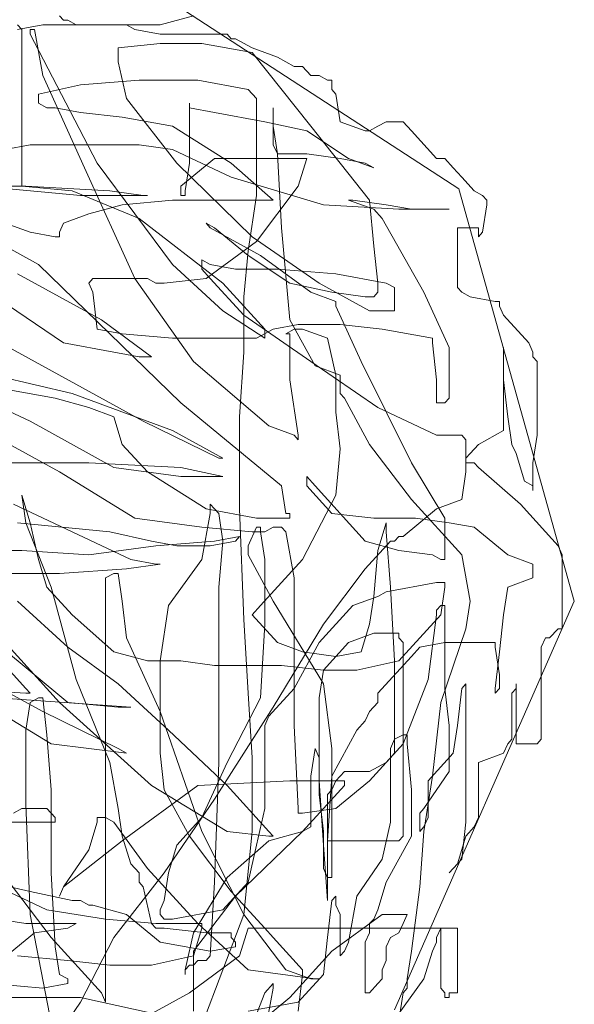
# Model space of a CAD drawing. Units: inches. Extents: x 1994 to 3075, y 3517 to 3950.
# Tile 41 of 58: x 1994.646332 to 1994.650517, y 3553.741889 to 3553.749313. Entities that reach past the tile are written whole.
import ezdxf

# ---------------------------------------------------------------- set-up
doc = ezdxf.new("R2010")
doc.units = ezdxf.units.IN
doc.layers.add('A-FURN-REFR', color=8, linetype='Continuous', lineweight=13)

msp = doc.modelspace()

# ---------------------------------------------------------------- linework, layer by layer
at = {"layer": 'A-FURN-REFR'}
for p, q in [((1994.6474175, 3553.7494858), (1994.6496449, 3553.7480373)), ((1994.6466639, 3553.7493078), (1994.6466323, 3553.7493426)), ((1994.6466955, 3553.7493078), (1994.6466639, 3553.7493078)), ((1994.6467587, 3553.7492731), (1994.6466955, 3553.7493078)), ((1994.6476438, 3553.7493426), (1994.647391, 3553.7492731)), ((1994.6463162, 3553.7492731), (1994.6463478, 3553.7492383)), ((1994.6465059, 3553.7492731), (1994.6463162, 3553.7492383)), ((1994.6463478, 3553.7492383), (1994.6463478, 3553.748057)), ((1994.6464111, 3553.7492383), (1994.6464427, 3553.7492383)), ((1994.6464111, 3553.7492037), (1994.6464111, 3553.7492383)), ((1994.6464427, 3553.7492383), (1994.6465059, 3553.7488909)), ((1994.647391, 3553.7492731), (1994.6465059, 3553.7492731)), ((1994.6471381, 3553.7492731), (1994.6467587, 3553.7492731)), ((1994.6472013, 3553.7492383), (1994.6471381, 3553.7492731)), ((1994.647391, 3553.7492037), (1994.6472013, 3553.7492383)), ((1994.6469168, 3553.7482307), (1994.6464111, 3553.7492037)), ((1994.6478967, 3553.7492037), (1994.647391, 3553.7492037)), ((1994.6479283, 3553.7491689), (1994.6478967, 3553.7492037)), ((1994.6479599, 3553.7491689), (1994.6479283, 3553.7491689)), ((1994.6480864, 3553.7490994), (1994.6479599, 3553.7491689)), ((1994.647391, 3553.7491341), (1994.6470749, 3553.7490994)), ((1994.6470749, 3553.7490994), (1994.6470749, 3553.7489951)), ((1994.647707, 3553.7491341), (1994.647391, 3553.7491341)), ((1994.6480864, 3553.7490646), (1994.647707, 3553.7491341)), ((1994.648276, 3553.7490299), (1994.6480864, 3553.7490994)), ((1994.6485289, 3553.7485087), (1994.6480864, 3553.7490646)), ((1994.6484025, 3553.7489604), (1994.648276, 3553.7490299)), ((1994.6470749, 3553.7489951), (1994.6471381, 3553.7487172)), ((1994.6484657, 3553.7489604), (1994.6484025, 3553.7489604)), ((1994.6485289, 3553.7488909), (1994.6484657, 3553.7489604)), ((1994.6465059, 3553.7488909), (1994.646822, 3553.7481959)), ((1994.6485921, 3553.7488909), (1994.6485289, 3553.7488909)), ((1994.6486553, 3553.7488562), (1994.6485921, 3553.7488909)), ((1994.6464743, 3553.7487519), (1994.6467904, 3553.7488214)), ((1994.6467904, 3553.7488214), (1994.6472329, 3553.7488562)), ((1994.6472329, 3553.7488562), (1994.6476754, 3553.7488562)), ((1994.6476754, 3553.7488562), (1994.6480548, 3553.7487867)), ((1994.6480548, 3553.7487867), (1994.648118, 3553.7487172)), ((1994.6486869, 3553.7488562), (1994.6486553, 3553.7488562)), ((1994.6486869, 3553.7487867), (1994.6486869, 3553.7488562)), ((1994.6487185, 3553.7487519), (1994.6486869, 3553.7487867)), ((1994.6464743, 3553.7486824), (1994.6464743, 3553.7487519)), ((1994.6471381, 3553.7487172), (1994.6475174, 3553.7482307)), ((1994.648118, 3553.7487172), (1994.648118, 3553.7479875)), ((1994.6487501, 3553.7485434), (1994.6487185, 3553.7487519)), ((1994.6465375, 3553.7486477), (1994.6464743, 3553.7486824)), ((1994.6466007, 3553.7486477), (1994.6465375, 3553.7486477)), ((1994.6467904, 3553.7486129), (1994.6466007, 3553.7486477)), ((1994.6476122, 3553.7486824), (1994.6476122, 3553.7482307)), ((1994.6476122, 3553.7486477), (1994.6476122, 3553.7486824)), ((1994.6478019, 3553.7486129), (1994.6476122, 3553.7486477)), ((1994.6482444, 3553.7486477), (1994.6482444, 3553.7483697)), ((1994.6482444, 3553.7485087), (1994.6482444, 3553.7486477)), ((1994.6471065, 3553.7485782), (1994.6467904, 3553.7486129)), ((1994.6474858, 3553.7485087), (1994.6471065, 3553.7485782)), ((1994.6481812, 3553.7485434), (1994.6478019, 3553.7486129)), ((1994.6479283, 3553.7482307), (1994.6474858, 3553.7485087)), ((1994.6484973, 3553.748474), (1994.6481812, 3553.7485434)), ((1994.648276, 3553.7483002), (1994.6482444, 3553.7485087)), ((1994.6489714, 3553.7479527), (1994.6485289, 3553.7485087)), ((1994.6489398, 3553.748474), (1994.6487501, 3553.7485434)), ((1994.6490347, 3553.7485087), (1994.6489714, 3553.748474)), ((1994.6490979, 3553.7485434), (1994.6490347, 3553.7485087)), ((1994.6492243, 3553.7485434), (1994.6490979, 3553.7485434)), ((1994.6492875, 3553.748474), (1994.6492243, 3553.7485434)), ((1994.6488134, 3553.7482654), (1994.6484973, 3553.748474)), ((1994.6489714, 3553.748474), (1994.6489398, 3553.748474)), ((1994.6494772, 3553.7482654), (1994.6492875, 3553.748474)), ((1994.6464111, 3553.7483697), (1994.6462214, 3553.7483349)), ((1994.6472329, 3553.7483697), (1994.6464111, 3553.7483697)), ((1994.6474858, 3553.7483349), (1994.6472329, 3553.7483697)), ((1994.6482444, 3553.7483697), (1994.648276, 3553.7483002)), ((1994.6479283, 3553.7481265), (1994.6474858, 3553.7483349)), ((1994.648276, 3553.7483002), (1994.6484973, 3553.7483002)), ((1994.6483076, 3553.7477443), (1994.648276, 3553.7483002)), ((1994.6484973, 3553.7483002), (1994.6487501, 3553.7482654)), ((1994.646822, 3553.7481959), (1994.6472013, 3553.747362)), ((1994.6474858, 3553.7474662), (1994.6469168, 3553.7482307)), ((1994.6475174, 3553.7482307), (1994.6480864, 3553.7476748)), ((1994.647549, 3553.748057), (1994.6478019, 3553.7482654)), ((1994.6476122, 3553.7482307), (1994.6475806, 3553.7480222)), ((1994.6478019, 3553.7482654), (1994.6484973, 3553.7482654)), ((1994.6482444, 3553.7479527), (1994.6479283, 3553.7482307)), ((1994.6484973, 3553.7482654), (1994.6484341, 3553.748057)), ((1994.6487501, 3553.7482654), (1994.6489398, 3553.7482307)), ((1994.649003, 3553.7481959), (1994.6488134, 3553.7482654)), ((1994.6489398, 3553.7482307), (1994.649003, 3553.7481959)), ((1994.6495404, 3553.7482654), (1994.6494772, 3553.7482654)), ((1994.6496036, 3553.7481959), (1994.6495404, 3553.7482654)), ((1994.6496669, 3553.7481265), (1994.6496036, 3553.7481959)), ((1994.6486237, 3553.747918), (1994.6479283, 3553.7481265)), ((1994.6497617, 3553.7480222), (1994.6496669, 3553.7481265)), ((1994.6451783, 3553.748057), (1994.6463794, 3553.748057)), ((1994.6467904, 3553.7479875), (1994.6460317, 3553.748057)), ((1994.6463478, 3553.748057), (1994.6467271, 3553.7480222)), ((1994.6463794, 3553.748057), (1994.6470116, 3553.7480222)), ((1994.647549, 3553.7479875), (1994.647549, 3553.748057)), ((1994.6484341, 3553.748057), (1994.648118, 3553.74764)), ((1994.6467271, 3553.7480222), (1994.6472329, 3553.7478137)), ((1994.6472961, 3553.7479875), (1994.6467904, 3553.7479875)), ((1994.6470116, 3553.7480222), (1994.6472645, 3553.7479875)), ((1994.6472645, 3553.7479875), (1994.6472961, 3553.7479875)), ((1994.6475806, 3553.7479875), (1994.647549, 3553.7479875)), ((1994.6475806, 3553.7480222), (1994.6475806, 3553.7479875)), ((1994.648118, 3553.7479875), (1994.6480548, 3553.7475705)), ((1994.6496449, 3553.7480373), (1994.6505167, 3553.7449295)), ((1994.6498249, 3553.7479875), (1994.6497617, 3553.7480222)), ((1994.6498565, 3553.7479527), (1994.6498249, 3553.7479875)), ((1994.6468536, 3553.7478485), (1994.6471065, 3553.747918)), ((1994.6471065, 3553.747918), (1994.6474858, 3553.7479527)), ((1994.6474858, 3553.7479527), (1994.6482444, 3553.7479527)), ((1994.6491927, 3553.7478832), (1994.6486237, 3553.747918)), ((1994.6488134, 3553.7479527), (1994.648845, 3553.7479527)), ((1994.649003, 3553.7478832), (1994.6488134, 3553.7479527)), ((1994.648845, 3553.7479527), (1994.6490979, 3553.747918)), ((1994.649003, 3553.7476053), (1994.6489714, 3553.7479527)), ((1994.6490979, 3553.747918), (1994.6492875, 3553.7478832)), ((1994.6498249, 3553.7477095), (1994.6498565, 3553.747918)), ((1994.6498565, 3553.747918), (1994.6498565, 3553.7479527)), ((1994.6457156, 3553.7478832), (1994.6464743, 3553.7474662)), ((1994.6466639, 3553.747779), (1994.6468536, 3553.7478485)), ((1994.6490663, 3553.7478137), (1994.649003, 3553.7478832)), ((1994.649572, 3553.7478832), (1994.6491927, 3553.7478832)), ((1994.6492875, 3553.7478832), (1994.649572, 3553.7478832)), ((1994.6462214, 3553.747779), (1994.6464111, 3553.7477095)), ((1994.6466323, 3553.7477095), (1994.6466639, 3553.747779)), ((1994.6472329, 3553.7478137), (1994.6478651, 3553.7473273)), ((1994.6477386, 3553.747779), (1994.6478019, 3553.7477443)), ((1994.6477703, 3553.7477443), (1994.6477386, 3553.747779)), ((1994.6493823, 3553.7472578), (1994.6490663, 3553.7478137)), ((1994.6464111, 3553.7477095), (1994.6466007, 3553.7476748)), ((1994.6466007, 3553.7476748), (1994.6466323, 3553.7476748)), ((1994.6466323, 3553.7476748), (1994.6466323, 3553.7477095)), ((1994.6481496, 3553.7475357), (1994.6477703, 3553.7477443)), ((1994.6478019, 3553.7477443), (1994.6480548, 3553.7475357)), ((1994.6480864, 3553.7476748), (1994.6485921, 3553.7473273)), ((1994.6483708, 3553.7470493), (1994.6483076, 3553.7477443)), ((1994.6496353, 3553.7477443), (1994.6497933, 3553.7477443)), ((1994.6496353, 3553.7472925), (1994.6496353, 3553.7477443)), ((1994.6497933, 3553.7477443), (1994.6497933, 3553.7476748)), ((1994.6497933, 3553.7476748), (1994.6498249, 3553.7477095)), ((1994.648118, 3553.74764), (1994.6477386, 3553.747362)), ((1994.6490347, 3553.7473273), (1994.649003, 3553.7476053)), ((1994.6480548, 3553.7475705), (1994.6480232, 3553.747223)), ((1994.6480548, 3553.7475357), (1994.6483708, 3553.7473273)), ((1994.6485289, 3553.7472578), (1994.6481496, 3553.7475357)), ((1994.6464743, 3553.7474662), (1994.647549, 3553.7464238)), ((1994.6478651, 3553.7471188), (1994.6474858, 3553.7474662)), ((1994.647707, 3553.747501), (1994.647707, 3553.7474316)), ((1994.6477703, 3553.7474662), (1994.647707, 3553.747501)), ((1994.6479599, 3553.7474316), (1994.6477703, 3553.7474662)), ((1994.6458421, 3553.7474316), (1994.6466639, 3553.7468756)), ((1994.6469484, 3553.7470493), (1994.6463162, 3553.7473968)), ((1994.647707, 3553.7474316), (1994.6477703, 3553.747362)), ((1994.648276, 3553.7474316), (1994.6479599, 3553.7474316)), ((1994.6487185, 3553.7473968), (1994.648276, 3553.7474316)), ((1994.6490979, 3553.7473273), (1994.6487185, 3553.7473968)), ((1994.6468852, 3553.747362), (1994.6468536, 3553.7473273)), ((1994.6468536, 3553.7473273), (1994.6468852, 3553.7472578)), ((1994.6472961, 3553.747362), (1994.6468852, 3553.747362)), ((1994.6472013, 3553.747362), (1994.6476438, 3553.7467365)), ((1994.6473593, 3553.7473273), (1994.6472961, 3553.747362)), ((1994.6474226, 3553.7473273), (1994.6473593, 3553.7473273)), ((1994.6477386, 3553.747362), (1994.6474226, 3553.7473273)), ((1994.6477703, 3553.747362), (1994.6480232, 3553.747084)), ((1994.6478651, 3553.7473273), (1994.6481812, 3553.7469798)), ((1994.6483708, 3553.7473273), (1994.6486869, 3553.7472578)), ((1994.6485921, 3553.7473273), (1994.6489714, 3553.7471188)), ((1994.6490347, 3553.7472578), (1994.6490347, 3553.7473273)), ((1994.6491611, 3553.7472925), (1994.6490979, 3553.7473273)), ((1994.6468852, 3553.7472578), (1994.6469168, 3553.7469798)), ((1994.6487185, 3553.7471883), (1994.6485289, 3553.7472578)), ((1994.6486869, 3553.7472578), (1994.6489398, 3553.747223)), ((1994.649003, 3553.747223), (1994.6490347, 3553.7472578)), ((1994.6491611, 3553.7471188), (1994.6491611, 3553.7472925)), ((1994.649572, 3553.7468408), (1994.6493823, 3553.7472578)), ((1994.6496669, 3553.7472578), (1994.6496353, 3553.7472925)), ((1994.6497301, 3553.747223), (1994.6496669, 3553.7472578)), ((1994.6480232, 3553.747223), (1994.6480232, 3553.7468061)), ((1994.6487185, 3553.7471535), (1994.6487185, 3553.7471883)), ((1994.6489082, 3553.7467365), (1994.6487185, 3553.7471535)), ((1994.6489398, 3553.747223), (1994.649003, 3553.747223)), ((1994.6499197, 3553.7471883), (1994.6497301, 3553.747223)), ((1994.6499513, 3553.7471883), (1994.6499197, 3553.7471883)), ((1994.6499513, 3553.7471535), (1994.6499513, 3553.7471883)), ((1994.6499829, 3553.747084), (1994.6499513, 3553.7471535)), ((1994.6481812, 3553.7469103), (1994.6478651, 3553.7471188)), ((1994.6480232, 3553.747084), (1994.6485289, 3553.7467365)), ((1994.6489714, 3553.7471188), (1994.6491611, 3553.7471188)), ((1994.6501726, 3553.7468756), (1994.6499829, 3553.747084)), ((1994.6473277, 3553.7467713), (1994.6469484, 3553.7470493)), ((1994.6482444, 3553.7469798), (1994.6484341, 3553.7470146)), ((1994.6485605, 3553.7467019), (1994.6483708, 3553.7470493)), ((1994.6484341, 3553.7470146), (1994.6487501, 3553.7470146)), ((1994.6487501, 3553.7470146), (1994.6490663, 3553.7469798)), ((1994.6469168, 3553.7469798), (1994.6471065, 3553.7469451)), ((1994.6471065, 3553.7469451), (1994.6474858, 3553.7469103)), ((1994.648118, 3553.7469103), (1994.6482444, 3553.7469798)), ((1994.6481812, 3553.7469798), (1994.6481812, 3553.7469103)), ((1994.6483392, 3553.7469451), (1994.6484025, 3553.7469798)), ((1994.6483708, 3553.7469451), (1994.6483392, 3553.7469451)), ((1994.6483708, 3553.7465976), (1994.6483708, 3553.7469451)), ((1994.6484025, 3553.7469798), (1994.6484657, 3553.7469798)), ((1994.6484657, 3553.7469798), (1994.6486553, 3553.7469103)), ((1994.6490663, 3553.7469798), (1994.6494456, 3553.7469103)), ((1994.6461265, 3553.7469103), (1994.6472645, 3553.7462849)), ((1994.6466639, 3553.7468756), (1994.6470433, 3553.7468061)), ((1994.6474858, 3553.7469103), (1994.648118, 3553.7469103)), ((1994.6486553, 3553.7469103), (1994.6487185, 3553.7466324)), ((1994.6494456, 3553.7469103), (1994.6494456, 3553.7468756)), ((1994.6494456, 3553.7468756), (1994.6494772, 3553.7465976)), ((1994.6502042, 3553.7468061), (1994.6501726, 3553.7468756)), ((1994.6470433, 3553.7468061), (1994.6472329, 3553.7467713)), ((1994.6480232, 3553.7468061), (1994.6479915, 3553.7463196)), ((1994.649572, 3553.7464586), (1994.649572, 3553.7468408)), ((1994.6499829, 3553.7468408), (1994.6499829, 3553.7465976)), ((1994.6499829, 3553.7462154), (1994.6499829, 3553.7468408)), ((1994.6502042, 3553.7467713), (1994.6502042, 3553.7468061)), ((1994.6472329, 3553.7467713), (1994.6473277, 3553.7467713)), ((1994.6476438, 3553.7467365), (1994.6482128, 3553.7462501)), ((1994.6485289, 3553.7467365), (1994.6490347, 3553.7463891)), ((1994.6492875, 3553.7459722), (1994.6489082, 3553.7467365)), ((1994.6502358, 3553.7467365), (1994.6502042, 3553.7467713)), ((1994.6502358, 3553.7461806), (1994.6502358, 3553.7467365)), ((1994.6467271, 3553.7464933), (1994.6458421, 3553.7467019)), ((1994.6487501, 3553.7466324), (1994.6485605, 3553.7467019)), ((1994.6484341, 3553.7461806), (1994.6483708, 3553.7465976)), ((1994.6487185, 3553.7466324), (1994.6487185, 3553.7463544)), ((1994.6487501, 3553.7464933), (1994.6487501, 3553.7466324)), ((1994.6494772, 3553.7465976), (1994.6494772, 3553.7464238)), ((1994.6499829, 3553.7465976), (1994.6500146, 3553.7463196)), ((1994.6459685, 3553.7464933), (1994.6464111, 3553.7462849)), ((1994.6466007, 3553.7464586), (1994.6462214, 3553.7465281)), ((1994.6474858, 3553.7462154), (1994.6467271, 3553.7464933)), ((1994.6487818, 3553.7464586), (1994.6487501, 3553.7464933)), ((1994.6468536, 3553.7463891), (1994.6466007, 3553.7464586)), ((1994.647549, 3553.7464238), (1994.6483076, 3553.7457984)), ((1994.6489714, 3553.7461111), (1994.6487818, 3553.7464586)), ((1994.6494772, 3553.7464238), (1994.6495404, 3553.7464238)), ((1994.6495404, 3553.7464238), (1994.649572, 3553.7464586)), ((1994.6470433, 3553.7463196), (1994.6468536, 3553.7463891)), ((1994.6487185, 3553.7463544), (1994.6487501, 3553.7460764)), ((1994.6490347, 3553.7463891), (1994.6494772, 3553.7461806)), ((1994.6464111, 3553.7462849), (1994.6470433, 3553.7459374)), ((1994.6471065, 3553.7461111), (1994.6470433, 3553.7463196)), ((1994.6472645, 3553.7462849), (1994.6478335, 3553.7460069)), ((1994.6479915, 3553.7463196), (1994.6479915, 3553.7456247)), ((1994.6500146, 3553.7463196), (1994.6500462, 3553.7461111)), ((1994.6478651, 3553.7460069), (1994.6474858, 3553.7462154)), ((1994.6482128, 3553.7462501), (1994.6484025, 3553.7461806)), ((1994.6497933, 3553.7461111), (1994.6499829, 3553.7462154)), ((1994.6461265, 3553.7461806), (1994.6466323, 3553.7459027)), ((1994.6484025, 3553.7461806), (1994.6484341, 3553.7461459)), ((1994.6484341, 3553.7461459), (1994.6484341, 3553.7461806)), ((1994.6494772, 3553.7461806), (1994.6496669, 3553.7461806)), ((1994.6496669, 3553.7461806), (1994.6496985, 3553.7461459)), ((1994.6496985, 3553.7461459), (1994.6496985, 3553.7459027)), ((1994.6502042, 3553.7459722), (1994.6502358, 3553.7461806)), ((1994.6472961, 3553.7459027), (1994.6471065, 3553.7461111)), ((1994.6487501, 3553.7460764), (1994.6487185, 3553.7457289)), ((1994.6492875, 3553.7456941), (1994.6489714, 3553.7461111)), ((1994.6496985, 3553.7460069), (1994.6497301, 3553.7460416)), ((1994.6497301, 3553.7460416), (1994.6497933, 3553.7461111)), ((1994.6500462, 3553.7461111), (1994.6500778, 3553.7460416)), ((1994.6500778, 3553.7460416), (1994.650141, 3553.7458332)), ((1994.6468536, 3553.7459722), (1994.6453996, 3553.7459722)), ((1994.647549, 3553.7459374), (1994.6468536, 3553.7459722)), ((1994.6478335, 3553.7460069), (1994.6478651, 3553.7460069)), ((1994.6495404, 3553.7455552), (1994.6492875, 3553.7459722)), ((1994.6496985, 3553.7459722), (1994.6496985, 3553.7460069)), ((1994.6497617, 3553.7459722), (1994.6496985, 3553.7459722)), ((1994.6497933, 3553.7459374), (1994.6497617, 3553.7459722)), ((1994.6502042, 3553.7457636), (1994.6502042, 3553.7459722)), ((1994.6466323, 3553.7459027), (1994.6472013, 3553.7455552)), ((1994.6470433, 3553.7459374), (1994.647549, 3553.7458679)), ((1994.6477386, 3553.7456247), (1994.6472961, 3553.7459027)), ((1994.6478651, 3553.7458679), (1994.647549, 3553.7459374)), ((1994.6496985, 3553.7459027), (1994.6496669, 3553.7456941)), ((1994.6501094, 3553.7456594), (1994.6497933, 3553.7459374)), ((1994.647549, 3553.7458679), (1994.6478651, 3553.7458679)), ((1994.6484973, 3553.7458679), (1994.6485605, 3553.7457984)), ((1994.6484973, 3553.7457984), (1994.6484973, 3553.7458679)), ((1994.650141, 3553.7458332), (1994.6502042, 3553.7457984)), ((1994.6483076, 3553.7457984), (1994.6483392, 3553.7455899)), ((1994.6486869, 3553.7455899), (1994.6484973, 3553.7457984)), ((1994.6485605, 3553.7457984), (1994.6487501, 3553.7455899)), ((1994.6502042, 3553.7457984), (1994.6502042, 3553.7457636)), ((1994.6463478, 3553.7457289), (1994.6463794, 3553.7455204)), ((1994.6464111, 3553.7455204), (1994.6463478, 3553.7457289)), ((1994.6487185, 3553.7457289), (1994.6484657, 3553.7452425)), ((1994.6496669, 3553.7452772), (1994.6492875, 3553.7456941)), ((1994.6496669, 3553.7456941), (1994.6494772, 3553.7456247)), ((1994.6462846, 3553.7456594), (1994.6471697, 3553.7452425)), ((1994.648118, 3553.7455552), (1994.6477386, 3553.7456247)), ((1994.6477703, 3553.7456594), (1994.6478335, 3553.7455899)), ((1994.6477703, 3553.7455899), (1994.6477703, 3553.7456594)), ((1994.6479915, 3553.7456247), (1994.6480232, 3553.7447907)), ((1994.6494772, 3553.7456247), (1994.6492243, 3553.7454162)), ((1994.650299, 3553.7454509), (1994.6501094, 3553.7456594)), ((1994.6463162, 3553.7455204), (1994.6470116, 3553.7454509)), ((1994.6463794, 3553.7455204), (1994.6465691, 3553.745034)), ((1994.6464743, 3553.7452425), (1994.6464111, 3553.7455204)), ((1994.6472013, 3553.7455552), (1994.647707, 3553.7454857)), ((1994.647707, 3553.7452425), (1994.6477703, 3553.7455899)), ((1994.6478335, 3553.7455899), (1994.6478651, 3553.7453814)), ((1994.6483708, 3553.7455552), (1994.648118, 3553.7455552)), ((1994.6483392, 3553.7455899), (1994.6483708, 3553.7455899)), ((1994.6483708, 3553.7455899), (1994.6483708, 3553.7455552)), ((1994.649003, 3553.7455552), (1994.6486869, 3553.7455899)), ((1994.6487501, 3553.7455899), (1994.6489398, 3553.7453814)), ((1994.6493191, 3553.7455552), (1994.649003, 3553.7455552)), ((1994.6490347, 3553.7453119), (1994.6490979, 3553.7455204)), ((1994.6490979, 3553.7455204), (1994.6490979, 3553.7454509)), ((1994.649572, 3553.7455204), (1994.6493191, 3553.7455552)), ((1994.6495404, 3553.7452425), (1994.6495404, 3553.7455552)), ((1994.6497617, 3553.7454857), (1994.649572, 3553.7455204)), ((1994.6470116, 3553.7454509), (1994.6473277, 3553.7453814)), ((1994.647707, 3553.7454857), (1994.6480864, 3553.7454509)), ((1994.6480548, 3553.7453467), (1994.648118, 3553.7454857)), ((1994.6480864, 3553.7454509), (1994.6481812, 3553.7454509)), ((1994.648118, 3553.7454857), (1994.6481496, 3553.7454857)), ((1994.6481496, 3553.7454857), (1994.6481496, 3553.7454509)), ((1994.6481496, 3553.7454509), (1994.6481812, 3553.7452425)), ((1994.6481812, 3553.7454509), (1994.6482444, 3553.7454857)), ((1994.6482444, 3553.7454857), (1994.6483076, 3553.7454857)), ((1994.6483076, 3553.7454857), (1994.6483392, 3553.7454509)), ((1994.6483392, 3553.7454509), (1994.6484025, 3553.7451035)), ((1994.6490979, 3553.7454509), (1994.6491295, 3553.745034)), ((1994.6500146, 3553.7452772), (1994.6497617, 3553.7454857)), ((1994.6503939, 3553.7453467), (1994.650299, 3553.7454509)), ((1994.6473277, 3553.7453814), (1994.6475174, 3553.7453467)), ((1994.6478019, 3553.7453814), (1994.6473593, 3553.7453467)), ((1994.6477703, 3553.7453467), (1994.6479599, 3553.7453814)), ((1994.6479915, 3553.7454162), (1994.6478019, 3553.7453814)), ((1994.6478651, 3553.7453814), (1994.6478335, 3553.745034)), ((1994.6479599, 3553.7453814), (1994.6479915, 3553.7454162)), ((1994.6491295, 3553.7453814), (1994.6489398, 3553.745173)), ((1994.6489398, 3553.7453814), (1994.6491927, 3553.7453119)), ((1994.6491611, 3553.7453814), (1994.6491295, 3553.7453814)), ((1994.6491927, 3553.7454162), (1994.6491611, 3553.7453814)), ((1994.6492243, 3553.7454162), (1994.6491927, 3553.7454162)), ((1994.6463478, 3553.7453119), (1994.6459053, 3553.7453119)), ((1994.6468536, 3553.7452772), (1994.6463478, 3553.7453119)), ((1994.6473593, 3553.7453467), (1994.6468536, 3553.7452772)), ((1994.6475174, 3553.7453467), (1994.6477703, 3553.7453467)), ((1994.6480548, 3553.7452772), (1994.6480548, 3553.7453467)), ((1994.649003, 3553.7449644), (1994.6490347, 3553.7453119)), ((1994.6491927, 3553.7453119), (1994.6494456, 3553.7452772)), ((1994.6504255, 3553.7452772), (1994.6503939, 3553.7453467)), ((1994.6465375, 3553.745034), (1994.6464743, 3553.7452425)), ((1994.6471697, 3553.7452425), (1994.6473593, 3553.7452077)), ((1994.6474542, 3553.744895), (1994.647707, 3553.7452425)), ((1994.6482444, 3553.7449298), (1994.6480548, 3553.7452772)), ((1994.6484657, 3553.7452425), (1994.6481496, 3553.744895)), ((1994.6481812, 3553.7452425), (1994.6481812, 3553.744756)), ((1994.6494456, 3553.7452772), (1994.6495088, 3553.7452425)), ((1994.6495088, 3553.7452425), (1994.6495404, 3553.7452425)), ((1994.6497301, 3553.7449298), (1994.6496669, 3553.7452772)), ((1994.6502042, 3553.7452077), (1994.6500146, 3553.7452772)), ((1994.6504255, 3553.7447212), (1994.6504255, 3553.7452772)), ((1994.6471381, 3553.745173), (1994.6466323, 3553.7451382)), ((1994.647391, 3553.7452077), (1994.6471381, 3553.745173)), ((1994.6473593, 3553.7452077), (1994.647391, 3553.7452077)), ((1994.6489398, 3553.745173), (1994.6486237, 3553.744756)), ((1994.6502042, 3553.7451035), (1994.6502042, 3553.7452077)), ((1994.6466323, 3553.7451382), (1994.6457472, 3553.7451382)), ((1994.64698, 3553.7451035), (1994.6470433, 3553.7451382)), ((1994.64698, 3553.7419067), (1994.64698, 3553.7451035)), ((1994.6470433, 3553.7451382), (1994.6470749, 3553.7451382)), ((1994.6470749, 3553.7451382), (1994.6471065, 3553.7449298)), ((1994.6484025, 3553.7451035), (1994.6484025, 3553.7439915)), ((1994.6500146, 3553.745034), (1994.6502042, 3553.7451035)), ((1994.6467271, 3553.7448255), (1994.6465375, 3553.745034)), ((1994.6465691, 3553.745034), (1994.6467587, 3553.744339)), ((1994.6478335, 3553.745034), (1994.6478335, 3553.7437136)), ((1994.6490979, 3553.7449992), (1994.6494772, 3553.7450687)), ((1994.6491295, 3553.745034), (1994.6491611, 3553.744478)), ((1994.6494772, 3553.7450687), (1994.6495404, 3553.7450687)), ((1994.6495404, 3553.745034), (1994.6495088, 3553.7448255)), ((1994.6495404, 3553.7450687), (1994.6495404, 3553.745034)), ((1994.6499829, 3553.7448255), (1994.6500146, 3553.745034)), ((1994.6459369, 3553.7449298), (1994.6466323, 3553.7441653)), ((1994.6466955, 3553.7445822), (1994.6463162, 3553.7449298)), ((1994.6471065, 3553.7449298), (1994.6471381, 3553.7446517)), ((1994.6486237, 3553.7443043), (1994.6482444, 3553.7449298)), ((1994.648845, 3553.744895), (1994.6490347, 3553.7449644)), ((1994.6489714, 3553.744756), (1994.649003, 3553.7449644)), ((1994.6490347, 3553.7449644), (1994.6490979, 3553.7449992)), ((1994.6505167, 3553.7449295), (1994.6491591, 3553.7418487)), ((1994.6496985, 3553.7447212), (1994.6497301, 3553.7449298)), ((1994.647391, 3553.744478), (1994.6474542, 3553.744895)), ((1994.6481496, 3553.744895), (1994.6480864, 3553.7448255)), ((1994.6485921, 3553.744617), (1994.648845, 3553.744895)), ((1994.6494772, 3553.7448603), (1994.6495088, 3553.744895)), ((1994.6494772, 3553.7448255), (1994.6494772, 3553.7448603)), ((1994.6495088, 3553.744895), (1994.6495404, 3553.744895)), ((1994.6495404, 3553.744895), (1994.6495404, 3553.7442695)), ((1994.6459369, 3553.7447907), (1994.6466955, 3553.7441653)), ((1994.6470433, 3553.7445475), (1994.6467271, 3553.7448255)), ((1994.6480232, 3553.7447907), (1994.6480548, 3553.7442348)), ((1994.6480864, 3553.7448255), (1994.648276, 3553.744617)), ((1994.6495088, 3553.7448255), (1994.6491927, 3553.744478)), ((1994.649414, 3553.744339), (1994.6494772, 3553.7448255)), ((1994.6499513, 3553.7445475), (1994.6499829, 3553.7448255)), ((1994.6481812, 3553.744756), (1994.6481496, 3553.7442001)), ((1994.6486237, 3553.744756), (1994.6482444, 3553.7441306)), ((1994.6489082, 3553.7445475), (1994.6489714, 3553.744756)), ((1994.6495088, 3553.7441653), (1994.6496985, 3553.7447212)), ((1994.6503306, 3553.7446517), (1994.6503939, 3553.7447212)), ((1994.6503939, 3553.7447212), (1994.6504255, 3553.7447212)), ((1994.6471381, 3553.7446517), (1994.647391, 3553.7440958)), ((1994.649003, 3553.7446865), (1994.6488134, 3553.744617)), ((1994.6491927, 3553.7446865), (1994.649003, 3553.7446865)), ((1994.6491927, 3553.7446517), (1994.6491927, 3553.7446865)), ((1994.6492243, 3553.744617), (1994.6491927, 3553.7446517)), ((1994.6502674, 3553.7445822), (1994.650299, 3553.7446517)), ((1994.650299, 3553.7446517), (1994.6503306, 3553.7446517)), ((1994.6470749, 3553.7443043), (1994.6466955, 3553.7445822)), ((1994.648276, 3553.744617), (1994.6484657, 3553.7445475)), ((1994.6484025, 3553.7442695), (1994.6485921, 3553.744617)), ((1994.6488134, 3553.744617), (1994.6486237, 3553.7444085)), ((1994.6492243, 3553.7431576), (1994.6492243, 3553.744617)), ((1994.6492875, 3553.7445128), (1994.6493507, 3553.7445822)), ((1994.6493507, 3553.7445822), (1994.6495404, 3553.744617)), ((1994.6495404, 3553.744617), (1994.6499197, 3553.744617)), ((1994.6499197, 3553.744617), (1994.6499197, 3553.7445822)), ((1994.6499197, 3553.7445822), (1994.6499513, 3553.7443738)), ((1994.6502674, 3553.7438873), (1994.6502674, 3553.7445822)), ((1994.6461265, 3553.7445475), (1994.6463794, 3553.7442695)), ((1994.6472961, 3553.744478), (1994.6470433, 3553.7445475)), ((1994.6484657, 3553.7445475), (1994.6487185, 3553.7445128)), ((1994.6487185, 3553.7445128), (1994.6489082, 3553.7445475)), ((1994.6490347, 3553.7442348), (1994.6492875, 3553.7445128)), ((1994.6499197, 3553.7442695), (1994.6499513, 3553.7445475)), ((1994.647549, 3553.744478), (1994.6472961, 3553.744478)), ((1994.647391, 3553.7437831), (1994.647391, 3553.744478)), ((1994.6478019, 3553.7444433), (1994.647549, 3553.744478)), ((1994.6483076, 3553.7444433), (1994.6478019, 3553.7444433)), ((1994.6486237, 3553.7444085), (1994.6483076, 3553.7444433)), ((1994.6486237, 3553.7444085), (1994.6485921, 3553.7442001)), ((1994.6488766, 3553.7444085), (1994.6486237, 3553.7444085)), ((1994.6491927, 3553.744478), (1994.6488766, 3553.7444085)), ((1994.6491611, 3553.744478), (1994.6491611, 3553.7437831)), ((1994.6460001, 3553.7443738), (1994.6465059, 3553.7440958)), ((1994.6467587, 3553.744339), (1994.6470116, 3553.7437136)), ((1994.6492243, 3553.7438526), (1994.649414, 3553.744339)), ((1994.6499513, 3553.7443738), (1994.6499513, 3553.7442695)), ((1994.6463794, 3553.7442348), (1994.6458105, 3553.7442695)), ((1994.6463794, 3553.7442695), (1994.6464111, 3553.7442348)), ((1994.6474542, 3553.7439568), (1994.6470749, 3553.7443043)), ((1994.6482128, 3553.7440611), (1994.6484025, 3553.7442695)), ((1994.6486869, 3553.7438178), (1994.6486237, 3553.7443043)), ((1994.6495404, 3553.7442695), (1994.649572, 3553.7439915)), ((1994.6496353, 3553.7439915), (1994.6496669, 3553.7442695)), ((1994.6496669, 3553.7442695), (1994.6496985, 3553.7443043)), ((1994.6496985, 3553.7443043), (1994.6496985, 3553.7432619)), ((1994.6499197, 3553.7442348), (1994.6499197, 3553.7442695)), ((1994.6499513, 3553.7442695), (1994.6499197, 3553.7442348)), ((1994.6500462, 3553.7442348), (1994.6500778, 3553.7442695)), ((1994.6500778, 3553.7443043), (1994.6500778, 3553.7438526)), ((1994.6500778, 3553.7442695), (1994.6500778, 3553.7443043)), ((1994.6465691, 3553.7438526), (1994.6460001, 3553.7442001)), ((1994.6471697, 3553.7441306), (1994.6461582, 3553.7442001)), ((1994.6464111, 3553.7442348), (1994.6463794, 3553.7442348)), ((1994.6464111, 3553.7441653), (1994.6464743, 3553.7442001)), ((1994.6464743, 3553.7442001), (1994.6465059, 3553.7442001)), ((1994.6465059, 3553.7442001), (1994.6465375, 3553.743922)), ((1994.6481496, 3553.7442001), (1994.6478967, 3553.7437136)), ((1994.6480548, 3553.7442348), (1994.6480864, 3553.7437483)), ((1994.6485921, 3553.7442001), (1994.6485921, 3553.7435746)), ((1994.6490347, 3553.7441653), (1994.6490347, 3553.7442348)), ((1994.6500462, 3553.7438873), (1994.6500462, 3553.7442348)), ((1994.6463794, 3553.7439568), (1994.6464111, 3553.7441653)), ((1994.6466323, 3553.7441653), (1994.6473277, 3553.7435398)), ((1994.6466955, 3553.7441653), (1994.6470749, 3553.7441306)), ((1994.6470749, 3553.7441306), (1994.6471697, 3553.7441306)), ((1994.6482444, 3553.7441306), (1994.6478019, 3553.7434356)), ((1994.6489714, 3553.7440958), (1994.6490347, 3553.7441653)), ((1994.6494456, 3553.7436093), (1994.6495088, 3553.7441653)), ((1994.6465059, 3553.7440958), (1994.6470749, 3553.7438178)), ((1994.647391, 3553.7440958), (1994.647707, 3553.7431923)), ((1994.6481812, 3553.7439915), (1994.6482128, 3553.7440611)), ((1994.6489398, 3553.7440263), (1994.6489714, 3553.7440958)), ((1994.6481812, 3553.7433661), (1994.6481812, 3553.7439915)), ((1994.6484025, 3553.7439915), (1994.6484341, 3553.7433661)), ((1994.6488766, 3553.7439568), (1994.6489398, 3553.7440263)), ((1994.649572, 3553.7439915), (1994.649572, 3553.7436441)), ((1994.6496036, 3553.7437831), (1994.6496353, 3553.7439915)), ((1994.6463794, 3553.7434009), (1994.6463794, 3553.7439568)), ((1994.6465375, 3553.743922), (1994.6465691, 3553.7435051)), ((1994.6478967, 3553.7435398), (1994.6474542, 3553.7439568)), ((1994.6486869, 3553.7436093), (1994.6488766, 3553.7439568)), ((1994.6491295, 3553.7438178), (1994.6491611, 3553.7438873)), ((1994.6491611, 3553.7438873), (1994.6492243, 3553.743922)), ((1994.6492243, 3553.743922), (1994.6492559, 3553.743922)), ((1994.6492559, 3553.743922), (1994.6492559, 3553.7438526)), ((1994.6500146, 3553.7438526), (1994.6500462, 3553.7438873)), ((1994.6502358, 3553.7438526), (1994.6502674, 3553.7438873)), ((1994.6471381, 3553.7437831), (1994.6465691, 3553.7438526)), ((1994.6470749, 3553.7438178), (1994.6471381, 3553.7437831)), ((1994.6485289, 3553.7436093), (1994.6485605, 3553.7438178)), ((1994.6485605, 3553.7438178), (1994.6485921, 3553.7437483)), ((1994.6486869, 3553.7428449), (1994.6486869, 3553.7438178)), ((1994.6489714, 3553.7435746), (1994.6492243, 3553.7438526)), ((1994.6491295, 3553.7432619), (1994.6491295, 3553.7438178)), ((1994.6492559, 3553.7438526), (1994.6492875, 3553.7435051)), ((1994.6499829, 3553.7437831), (1994.6500146, 3553.7438526)), ((1994.6500778, 3553.7438526), (1994.6502358, 3553.7438526)), ((1994.6474226, 3553.7435051), (1994.647391, 3553.7437831)), ((1994.6480864, 3553.7437483), (1994.6480864, 3553.7431923)), ((1994.6485921, 3553.7437483), (1994.6485921, 3553.7434704)), ((1994.6491611, 3553.7437831), (1994.6490979, 3553.7437136)), ((1994.649414, 3553.7435746), (1994.6496036, 3553.7437831)), ((1994.6497933, 3553.7437136), (1994.6499829, 3553.7437831)), ((1994.6470116, 3553.7437136), (1994.6470749, 3553.7433661)), ((1994.6478967, 3553.7437136), (1994.647707, 3553.7432966)), ((1994.6478335, 3553.7437136), (1994.6478019, 3553.7428101)), ((1994.6490979, 3553.7437136), (1994.6489714, 3553.7436441)), ((1994.6497933, 3553.7432966), (1994.6497933, 3553.7437136)), ((1994.6485289, 3553.7432271), (1994.6485289, 3553.7436093)), ((1994.6486553, 3553.7431229), (1994.6486869, 3553.7436093)), ((1994.6487818, 3553.7436441), (1994.6487185, 3553.7435746)), ((1994.6489714, 3553.7436441), (1994.6487818, 3553.7436441)), ((1994.649572, 3553.7436441), (1994.6493823, 3553.7433661)), ((1994.6493823, 3553.7431923), (1994.6494456, 3553.7436093)), ((1994.6471065, 3553.7431229), (1994.6476754, 3553.7435398)), ((1994.6473277, 3553.7435398), (1994.6478967, 3553.7431923)), ((1994.6476754, 3553.7435398), (1994.6483708, 3553.7435746)), ((1994.6482128, 3553.7431923), (1994.6478967, 3553.7435398)), ((1994.6483708, 3553.7435746), (1994.6487818, 3553.7435746)), ((1994.6487818, 3553.7435398), (1994.6484657, 3553.7431923)), ((1994.6485921, 3553.7435746), (1994.6486237, 3553.7430882)), ((1994.6487185, 3553.7435746), (1994.6486869, 3553.7435051)), ((1994.6487185, 3553.7433661), (1994.6489714, 3553.7435746)), ((1994.6487818, 3553.7435746), (1994.6487818, 3553.7435398)), ((1994.649414, 3553.7432966), (1994.649414, 3553.7435746)), ((1994.6465691, 3553.7435051), (1994.6465691, 3553.7428796)), ((1994.6476122, 3553.7431576), (1994.6474226, 3553.7435051)), ((1994.6485921, 3553.7434704), (1994.6486237, 3553.7431923)), ((1994.6486869, 3553.7435051), (1994.6486553, 3553.7434704)), ((1994.6486553, 3553.7434704), (1994.6486553, 3553.7431229)), ((1994.6492875, 3553.7435051), (1994.6492875, 3553.7431576)), ((1994.6464111, 3553.7425669), (1994.6463794, 3553.7434009)), ((1994.6478019, 3553.7434356), (1994.6474226, 3553.7428796)), ((1994.6463478, 3553.7433661), (1994.6462846, 3553.7433314)), ((1994.6465375, 3553.7433661), (1994.6463478, 3553.7433661)), ((1994.6466007, 3553.7432966), (1994.6465375, 3553.7433661)), ((1994.6466007, 3553.7432619), (1994.6466007, 3553.7432966)), ((1994.6469168, 3553.7432966), (1994.6469168, 3553.7432619)), ((1994.64698, 3553.7432966), (1994.6469168, 3553.7432966)), ((1994.6470433, 3553.7432619), (1994.64698, 3553.7432966)), ((1994.6470749, 3553.7433661), (1994.6471065, 3553.7431576)), ((1994.647707, 3553.7432966), (1994.6475174, 3553.7430882)), ((1994.648118, 3553.7430882), (1994.6481812, 3553.7433661)), ((1994.6484341, 3553.7433661), (1994.6484341, 3553.7433314)), ((1994.6484341, 3553.7433314), (1994.6484657, 3553.7433314)), ((1994.6484657, 3553.7433314), (1994.6487185, 3553.7433661)), ((1994.6493823, 3553.7433661), (1994.6493507, 3553.7433314)), ((1994.6493507, 3553.7433314), (1994.6493507, 3553.7431923)), ((1994.6493823, 3553.7432271), (1994.649414, 3553.7432966)), ((1994.6497617, 3553.7432271), (1994.6497933, 3553.7432966)), ((1994.6456524, 3553.7432619), (1994.6466007, 3553.7432619)), ((1994.6469168, 3553.7432619), (1994.6468536, 3553.7430534)), ((1994.6472961, 3553.7429144), (1994.6470433, 3553.7432619)), ((1994.6484657, 3553.7431923), (1994.6485289, 3553.7432271)), ((1994.6490663, 3553.7429839), (1994.6491295, 3553.7432619)), ((1994.6493507, 3553.7431923), (1994.6493823, 3553.7432271)), ((1994.6496985, 3553.7432619), (1994.6496669, 3553.7429839)), ((1994.6496985, 3553.7431576), (1994.6497617, 3553.7432271)), ((1994.6471065, 3553.7431576), (1994.6471697, 3553.7429491)), ((1994.6479283, 3553.7427407), (1994.6476122, 3553.7431576)), ((1994.647707, 3553.7431923), (1994.6480232, 3553.7425669)), ((1994.6478967, 3553.7431923), (1994.6482128, 3553.7431576)), ((1994.6484657, 3553.7431923), (1994.6479599, 3553.7427059)), ((1994.6480864, 3553.7431923), (1994.6480232, 3553.7425669)), ((1994.6482444, 3553.7431576), (1994.6482128, 3553.7431923)), ((1994.6482128, 3553.7431229), (1994.6484657, 3553.7431923)), ((1994.6482128, 3553.7431576), (1994.6482444, 3553.7431576)), ((1994.6486237, 3553.7431923), (1994.6486237, 3553.7429144)), ((1994.6492875, 3553.7431576), (1994.6490979, 3553.7428101)), ((1994.6491927, 3553.7431229), (1994.6492243, 3553.7431576)), ((1994.6493507, 3553.7427754), (1994.6493823, 3553.7431923)), ((1994.6496353, 3553.7429491), (1994.6496985, 3553.7431576)), ((1994.6466639, 3553.7427754), (1994.6471065, 3553.7431229)), ((1994.6475174, 3553.7430882), (1994.6474542, 3553.7428796)), ((1994.6478967, 3553.7428449), (1994.6482128, 3553.7431229)), ((1994.6480548, 3553.7428101), (1994.648118, 3553.7430882)), ((1994.6486237, 3553.7430882), (1994.6486553, 3553.7426712)), ((1994.6486553, 3553.7426712), (1994.6486553, 3553.7431229)), ((1994.6486553, 3553.7431229), (1994.6491927, 3553.7431229)), ((1994.6468536, 3553.7430534), (1994.6466639, 3553.7427754)), ((1994.6471697, 3553.7429491), (1994.6472329, 3553.7428796)), ((1994.6488766, 3553.7427059), (1994.6490663, 3553.7429839)), ((1994.649572, 3553.7428796), (1994.6496353, 3553.7429491)), ((1994.6496669, 3553.7429839), (1994.6496036, 3553.7429144)), ((1994.6465691, 3553.7428796), (1994.6466007, 3553.7423237)), ((1994.6474226, 3553.7428796), (1994.6470433, 3553.7423932)), ((1994.6472329, 3553.7428796), (1994.6472329, 3553.7428101)), ((1994.6476754, 3553.7424974), (1994.6472961, 3553.7429144)), ((1994.6474542, 3553.7428796), (1994.6474226, 3553.7426712)), ((1994.6486237, 3553.7429144), (1994.6486553, 3553.7428449)), ((1994.6496036, 3553.7429144), (1994.649572, 3553.7428796)), ((1994.6460949, 3553.7428101), (1994.6465375, 3553.7426017)), ((1994.6464111, 3553.7427407), (1994.6460949, 3553.7428101)), ((1994.646253, 3553.7428101), (1994.6465691, 3553.7423932)), ((1994.6466323, 3553.7427059), (1994.6466639, 3553.7427754)), ((1994.6466639, 3553.7427754), (1994.6466323, 3553.7427059)), ((1994.6472329, 3553.7428101), (1994.6472645, 3553.7427754)), ((1994.6472645, 3553.7427754), (1994.6473277, 3553.7424974)), ((1994.6476438, 3553.742428), (1994.6478967, 3553.7428449)), ((1994.6478019, 3553.7428101), (1994.6477703, 3553.7422542)), ((1994.6478651, 3553.7426017), (1994.6480548, 3553.7428101)), ((1994.6486553, 3553.7428449), (1994.6486869, 3553.7428449)), ((1994.6490979, 3553.7428101), (1994.6490347, 3553.7426017)), ((1994.6492875, 3553.742289), (1994.6493507, 3553.7427754)), ((1994.6467271, 3553.7426712), (1994.6464111, 3553.7427407)), ((1994.6479599, 3553.7427059), (1994.6476438, 3553.742289)), ((1994.6481812, 3553.7424627), (1994.6479283, 3553.7427407)), ((1994.6486869, 3553.7426712), (1994.6487185, 3553.7427059)), ((1994.6487185, 3553.7427059), (1994.6487185, 3553.7426364)), ((1994.6488134, 3553.7423585), (1994.6488766, 3553.7427059)), ((1994.6467904, 3553.7426712), (1994.6467271, 3553.7426712)), ((1994.6468536, 3553.7426364), (1994.6467904, 3553.7426712)), ((1994.6468852, 3553.7426364), (1994.6468536, 3553.7426364)), ((1994.6471381, 3553.7425669), (1994.6468852, 3553.7426364)), ((1994.6474226, 3553.7426712), (1994.647391, 3553.7426017)), ((1994.6486553, 3553.7423932), (1994.6486869, 3553.7426712)), ((1994.6487185, 3553.7426364), (1994.6487501, 3553.7425669)), ((1994.6463794, 3553.7424974), (1994.6459369, 3553.7425669)), ((1994.6466007, 3553.741594), (1994.6464111, 3553.7425669)), ((1994.6465375, 3553.7426017), (1994.64698, 3553.7425322)), ((1994.647391, 3553.7423585), (1994.6471381, 3553.7425669)), ((1994.647391, 3553.7426017), (1994.647391, 3553.7425669)), ((1994.647391, 3553.7425669), (1994.6474226, 3553.7425322)), ((1994.6474858, 3553.7425322), (1994.6478651, 3553.7426017)), ((1994.6480232, 3553.7425669), (1994.647707, 3553.741733)), ((1994.6480232, 3553.7425669), (1994.6483392, 3553.7421499)), ((1994.6490663, 3553.7425669), (1994.6486869, 3553.742289)), ((1994.6487501, 3553.7425669), (1994.6487501, 3553.7422542)), ((1994.6490347, 3553.7426017), (1994.649003, 3553.7425322)), ((1994.6492559, 3553.7425669), (1994.6490663, 3553.7425669)), ((1994.6492243, 3553.7424974), (1994.6492559, 3553.7425669)), ((1994.6467587, 3553.7424974), (1994.6463794, 3553.7424974)), ((1994.6466955, 3553.7424627), (1994.6467587, 3553.7424974)), ((1994.64698, 3553.7425322), (1994.6473593, 3553.7424974)), ((1994.6473277, 3553.7424974), (1994.6473593, 3553.7424627)), ((1994.6473593, 3553.7424974), (1994.647707, 3553.7424974)), ((1994.6474226, 3553.7425322), (1994.6474858, 3553.7425322)), ((1994.6480548, 3553.7421499), (1994.6476754, 3553.7424974)), ((1994.647707, 3553.7424974), (1994.647707, 3553.7424627)), ((1994.649003, 3553.7425322), (1994.6489714, 3553.7424974)), ((1994.6489714, 3553.7424974), (1994.6489714, 3553.742428)), ((1994.6491927, 3553.742428), (1994.6492243, 3553.7424974)), ((1994.6461898, 3553.7422194), (1994.6464427, 3553.742428)), ((1994.6464427, 3553.742428), (1994.6466955, 3553.7424627)), ((1994.6473593, 3553.7424627), (1994.6474226, 3553.7424627)), ((1994.6474226, 3553.7424627), (1994.6477386, 3553.742428)), ((1994.6475806, 3553.7421499), (1994.6476438, 3553.742428)), ((1994.647707, 3553.7424627), (1994.6476438, 3553.7422542)), ((1994.6477386, 3553.742428), (1994.6479283, 3553.742428)), ((1994.6479283, 3553.742428), (1994.6479283, 3553.7423932)), ((1994.6480548, 3553.7424627), (1994.6479915, 3553.7422542)), ((1994.6496353, 3553.7424627), (1994.6480548, 3553.7424627)), ((1994.6482444, 3553.7423932), (1994.6481812, 3553.7424627)), ((1994.6489714, 3553.742428), (1994.6489398, 3553.7423585)), ((1994.6491295, 3553.7423932), (1994.6491927, 3553.742428)), ((1994.6494772, 3553.7423932), (1994.6495088, 3553.7424627)), ((1994.6495088, 3553.7424627), (1994.6495088, 3553.742011)), ((1994.6496353, 3553.7419762), (1994.6496353, 3553.7424627)), ((1994.6465691, 3553.7423932), (1994.6469484, 3553.7419762)), ((1994.6470433, 3553.7423932), (1994.6467904, 3553.7419067)), ((1994.6477703, 3553.742289), (1994.647391, 3553.7423585)), ((1994.6479283, 3553.7423932), (1994.6479599, 3553.7423585)), ((1994.6479599, 3553.7423585), (1994.6479599, 3553.7423237)), ((1994.6484657, 3553.7421499), (1994.6482444, 3553.7423932)), ((1994.6486237, 3553.7421152), (1994.6486553, 3553.7423932)), ((1994.6487818, 3553.742289), (1994.6488134, 3553.7423585)), ((1994.6489398, 3553.7423585), (1994.6489398, 3553.7419762)), ((1994.6490979, 3553.7423237), (1994.6491295, 3553.7423932)), ((1994.6494456, 3553.742289), (1994.6494772, 3553.7423585)), ((1994.6494772, 3553.7423585), (1994.6494772, 3553.7423932)), ((1994.6466955, 3553.7422194), (1994.6463162, 3553.7422542)), ((1994.6466007, 3553.7423237), (1994.6466323, 3553.7421152)), ((1994.6476438, 3553.7422542), (1994.6473277, 3553.7421847)), ((1994.6479915, 3553.7422542), (1994.6476122, 3553.7419762)), ((1994.6476438, 3553.742289), (1994.6476438, 3553.7418372)), ((1994.6477703, 3553.7422542), (1994.6477386, 3553.7422194)), ((1994.6479599, 3553.7423237), (1994.6477703, 3553.742289)), ((1994.6486869, 3553.742289), (1994.6483708, 3553.7419415)), ((1994.6487501, 3553.7422542), (1994.6487818, 3553.742289)), ((1994.6490979, 3553.7422194), (1994.6490979, 3553.7423237)), ((1994.6492559, 3553.7420804), (1994.6492875, 3553.742289)), ((1994.6493823, 3553.7420804), (1994.6494456, 3553.742289)), ((1994.6470116, 3553.7421847), (1994.6466955, 3553.7422194)), ((1994.6473277, 3553.7421847), (1994.6470116, 3553.7421847)), ((1994.6476122, 3553.7421847), (1994.6475806, 3553.7421499)), ((1994.6476438, 3553.7421847), (1994.6476122, 3553.7421847)), ((1994.6476754, 3553.7422194), (1994.6476438, 3553.7421847)), ((1994.6477386, 3553.7422194), (1994.6476754, 3553.7422194)), ((1994.6490663, 3553.7421499), (1994.6490979, 3553.7422194)), ((1994.6466323, 3553.7421152), (1994.6466955, 3553.7420804)), ((1994.6475806, 3553.7421152), (1994.6475806, 3553.7421499)), ((1994.6475806, 3553.7421499), (1994.6475806, 3553.7421152)), ((1994.6485605, 3553.7420804), (1994.6480548, 3553.7421499)), ((1994.6483392, 3553.7421499), (1994.6485289, 3553.7420804)), ((1994.6484341, 3553.7418372), (1994.6484657, 3553.7421152)), ((1994.6484341, 3553.7419067), (1994.6486237, 3553.7421152)), ((1994.6484657, 3553.7421152), (1994.6484657, 3553.7421499)), ((1994.6490663, 3553.7420804), (1994.6490663, 3553.7421499)), ((1994.6465059, 3553.742011), (1994.6461265, 3553.7420457)), ((1994.6466955, 3553.7420457), (1994.6465059, 3553.742011)), ((1994.6466955, 3553.7420804), (1994.6466955, 3553.7420457)), ((1994.6481812, 3553.7419762), (1994.6482444, 3553.7420457)), ((1994.6482444, 3553.7420457), (1994.6482444, 3553.742011)), ((1994.6485289, 3553.7420804), (1994.6485921, 3553.7420804)), ((1994.6485921, 3553.7420804), (1994.6485605, 3553.7420804)), ((1994.6489714, 3553.7419762), (1994.6490347, 3553.7420457)), ((1994.6490347, 3553.7420457), (1994.6490663, 3553.7420804)), ((1994.6491295, 3553.741733), (1994.6493823, 3553.7420804)), ((1994.6492559, 3553.742011), (1994.6492559, 3553.7420804)), ((1994.6469484, 3553.7419762), (1994.64698, 3553.7419067)), ((1994.6476122, 3553.7419762), (1994.6472329, 3553.7417677)), ((1994.6479915, 3553.7414898), (1994.6481812, 3553.7419762)), ((1994.6482444, 3553.742011), (1994.6481812, 3553.7416635)), ((1994.6489398, 3553.7419762), (1994.6489714, 3553.7419762)), ((1994.6491927, 3553.7417677), (1994.6492243, 3553.7419762)), ((1994.6492243, 3553.7419762), (1994.6492559, 3553.742011)), ((1994.6495088, 3553.742011), (1994.6495404, 3553.7419762)), ((1994.6495404, 3553.7419762), (1994.6495404, 3553.7419415)), ((1994.649572, 3553.7419762), (1994.6496353, 3553.7419762)), ((1994.649572, 3553.7419415), (1994.649572, 3553.7419762)), ((1994.6458421, 3553.7419415), (1994.6467904, 3553.7419415)), ((1994.6467904, 3553.7419067), (1994.6466007, 3553.7416288)), ((1994.6467904, 3553.7419415), (1994.6477386, 3553.741733)), ((1994.6480548, 3553.7418372), (1994.6484341, 3553.7419067)), ((1994.6483708, 3553.7419415), (1994.648118, 3553.741733)), ((1994.6495404, 3553.7419415), (1994.649572, 3553.7419415))]:
    msp.add_line(p, q, dxfattribs=at)

doc.saveas('drawing.dxf')
